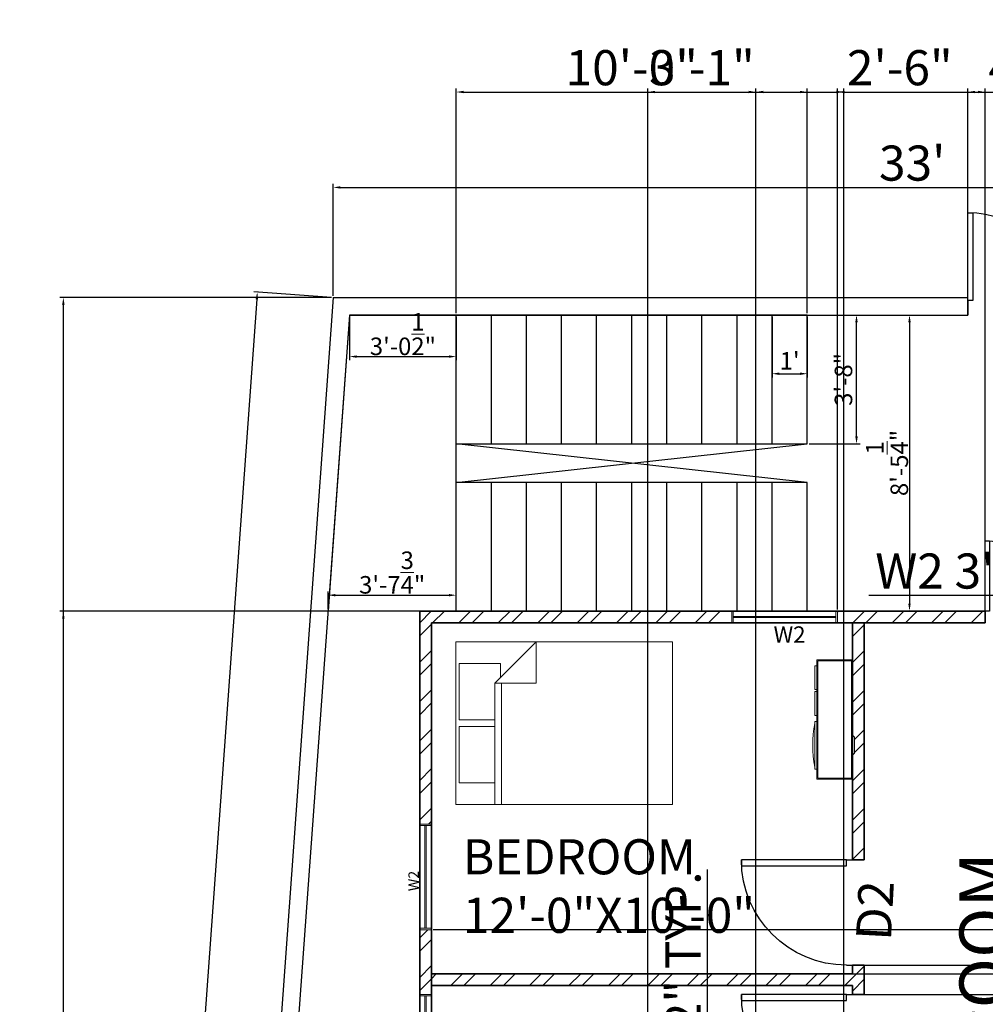
# Model space of a CAD drawing. Units: inches. Extents: x 2242 to 2870, y 1782 to 2635.
# Tile 6 of 7: x 2252 to 2582, y 2299 to 2635. Entities that reach past the tile are written whole.
import ezdxf

# ---------------------------------------------------------------- set-up
doc = ezdxf.new("R2010")
doc.units = ezdxf.units.IN
for name, color, linetype, lineweight in [('A-ANNO-DIMS', 7, 'Continuous', 18), ('A-ANNO-TEXT', 1, 'Continuous', 18), ('A-AREA-IDEN', 1, 'Continuous', 25), ('A-WALL-PATT', 253, 'Continuous', 13), ('C-PROP', 7, 'Continuous', 30), ('doors', 5, 'Continuous', 25), ('furniture', 9, 'Continuous', 18), ('stair case', 6, 'Continuous', 25), ('walls', 7, 'Continuous', 35), ('windows', 72, 'Continuous', 18)]:
    doc.layers.add(name, color=color, linetype=linetype, lineweight=lineweight)
doc.styles.get("Standard").update_dxf_attribs({"font": 'arial.ttf'})
doc.dimstyles.new('ISO-25', dxfattribs={"dimtxt": 12, "dimasz": 2.5, "dimexe": 1.25, "dimexo": 0.625, "dimtad": 1, "dimlunit": 4, "dimtxsty": 'Standard', "dimcen": 2.5, "dimadec": 0, "dimazin": 0, "dimtfac": 1, "dimtmove": 0, "dimatfit": 3, "dimfxl": 1, "dimarcsym": 0})

# ---------------------------------------------------------------- blocks, each defined once
blk = doc.blocks.new('*U2')
for p, q in [((0, 0), (0, -5)), ((30, 0), (30, -5))]:
    blk.add_line(p, q)
blk.add_lwpolyline([(0, 0), (0, 30), (1.75, 30), (1.75, 0)], close=True)
blk.add_arc((0, 0), 30, 0, 90)
blk = doc.blocks.new('Bed - Queen')
for p, q in [((0, -80.00003), (0, 0)), ((0, 0), (59.99999, 0)), ((59.99999, 0), (59.99999, -80.00003)), ((7.99999, -1.2), (28.79998, -1.2)), ((7.99999, -14.4), (7.99999, -1.2)), ((28.79998, -1.2), (28.79998, -14.4)), ((31.19999, -1.2), (51.99999, -1.2)), ((31.19999, -14.4), (31.19999, -1.2)), ((51.99999, -1.2), (51.99999, -16.4)), ((0, -14.4), (44.8, -14.4)), ((59.99999, -29.6), (44.8, -14.4)), ((44.8, -14.4), (44.8, -29.6)), ((44.8, -16.8), (0, -16.8)), ((51.99999, -16.4), (46.79936, -16.4)), ((44.8, -29.6), (59.99999, -29.6)), ((59.99999, -80.00003), (0, -80.00003))]:
    blk.add_line(p, q)
blk = doc.blocks.new('Entertainment Center')
for p, q in [((-4, 0), (-5, -1)), ((4, 0), (-4, 0)), ((5, -1), (4, 0)), ((-17, -19), (-17, -1)), ((-17, -1), (43, -1)), ((-16.5, -18.5), (-16.5, -1.5)), ((-16.5, -1.5), (42.5, -1.5)), ((42.5, -1.5), (42.5, -18.5)), ((43, -1), (43, -19)), ((43, -19), (-17, -19)), ((42.5, -18.5), (-16.5, -18.5)), ((-12, -20), (-12, -19)), ((12, -19), (12, -20)), ((15, -20), (15, -19)), ((27, -19), (27, -20)), ((28, -20), (28, -19)), ((40, -19), (40, -20)), ((12, -20), (-12, -20)), ((27, -20), (15, -20)), ((40, -20), (28, -20))]:
    blk.add_line(p, q)
blk.add_arc((0, 40), 61, 259.6111, 280.3889)
blk = doc.blocks.new('*D15')
at = {"layer": 'A-ANNO-DIMS', "color": 0, "lineweight": -2, "transparency": 16777216}
for p, q in [((2359.16, 2540.96), (2359.16, 2579.23)), ((2755.16, 2540.96), (2755.16, 2579.23)), ((2361.66, 2577.98), (2752.66, 2577.98))]:
    blk.add_line(p, q, dxfattribs=at)
at = {"layer": 'A-ANNO-DIMS', "color": 0, "transparency": 16777216}
for points in [[(2361.66, 2578.39), (2361.66, 2577.56), (2359.16, 2577.98)], [(2752.66, 2578.39), (2752.66, 2577.56), (2755.16, 2577.98)]]:
    blk.add_solid(points, dxfattribs=at)
at = {"layer": 'Defpoints', "color": 0, "transparency": 16777216}
for p in [(2755.16, 2577.98), (2359.16, 2540.33), (2755.16, 2540.33)]:
    blk.add_point(p, dxfattribs=at)
at = {"layer": 'A-ANNO-DIMS', "color": 0, "transparency": 16777216, "insert": (2557.16, 2584.73), "char_height": 12, "attachment_point": 5}
blk.add_mtext("33'", dxfattribs=at)
blk = doc.blocks.new('*D16')
at = {"layer": 'A-ANNO-DIMS', "color": 0, "lineweight": -2, "transparency": 16777216}
for p, q in [((2358.54, 2540.38), (2331.98, 2542.3)), ((2333.04, 2539.72), (2282.38, 1840.55)), ((2307.51, 1836.23), (2280.95, 1838.15))]:
    blk.add_line(p, q, dxfattribs=at)
at = {"layer": 'A-ANNO-DIMS', "color": 0, "transparency": 16777216}
for points in [[(2332.63, 2539.75), (2333.46, 2539.69), (2333.22, 2542.21)], [(2281.96, 1840.58), (2282.79, 1840.52), (2282.2, 1838.06)]]:
    blk.add_solid(points, dxfattribs=at)
at = {"layer": 'Defpoints', "color": 0, "transparency": 16777216}
for p in [(2359.16, 2540.33), (2282.2, 1838.06), (2308.14, 1836.18)]:
    blk.add_point(p, dxfattribs=at)
at = {"layer": 'A-ANNO-DIMS', "color": 0, "transparency": 16777216, "insert": (2300.98, 2190.63), "char_height": 12, "attachment_point": 5, "rotation": 85.8553}
blk.add_mtext('58\'-10"', dxfattribs=at)
blk = doc.blocks.new('*D23')
at = {"layer": 'A-ANNO-DIMS', "color": 0, "lineweight": -2, "transparency": 16777216}
for p, q in [((2509.25, 2533.71), (2509.25, 2513.03)), ((2521.25, 2533.71), (2521.25, 2513.03)), ((2511.75, 2514.28), (2518.75, 2514.28))]:
    blk.add_line(p, q, dxfattribs=at)
at = {"layer": 'A-ANNO-DIMS', "color": 0, "transparency": 16777216}
for points in [[(2511.75, 2514.7), (2511.75, 2513.86), (2509.25, 2514.28)], [(2518.75, 2514.7), (2518.75, 2513.86), (2521.25, 2514.28)]]:
    blk.add_solid(points, dxfattribs=at)
at = {"layer": 'Defpoints', "color": 0, "transparency": 16777216}
for p in [(2509.25, 2534.33), (2521.25, 2534.33), (2521.25, 2514.28)]:
    blk.add_point(p, dxfattribs=at)
at = {"layer": 'A-ANNO-DIMS', "color": 0, "transparency": 16777216, "insert": (2515.25, 2517.92), "char_height": 6, "attachment_point": 5}
blk.add_mtext("1'", dxfattribs=at)
blk = doc.blocks.new('*D24')
at = {"layer": 'A-ANNO-DIMS', "color": 0, "lineweight": -2, "transparency": 16777216}
for p, q in [((2521.88, 2534.33), (2539.37, 2534.33)), ((2538.12, 2492.83), (2538.12, 2531.83)), ((2521.88, 2490.33), (2539.37, 2490.33))]:
    blk.add_line(p, q, dxfattribs=at)
at = {"layer": 'A-ANNO-DIMS', "color": 0, "transparency": 16777216}
for points in [[(2537.7, 2531.83), (2538.54, 2531.83), (2538.12, 2534.33)], [(2537.7, 2492.83), (2538.54, 2492.83), (2538.12, 2490.33)]]:
    blk.add_solid(points, dxfattribs=at)
at = {"layer": 'Defpoints', "color": 0, "transparency": 16777216}
for p in [(2521.25, 2534.33), (2538.12, 2534.33), (2521.25, 2490.33)]:
    blk.add_point(p, dxfattribs=at)
at = {"layer": 'A-ANNO-DIMS', "color": 0, "transparency": 16777216, "insert": (2534.43, 2512.33), "char_height": 6, "attachment_point": 5, "rotation": 90}
blk.add_mtext('3\'-8"', dxfattribs=at)
blk = doc.blocks.new('*D25')
at = {"layer": 'A-ANNO-DIMS', "color": 0, "lineweight": -2, "transparency": 16777216}
for p, q in [((2521.88, 2534.33), (2557.49, 2534.33)), ((2556.24, 2531.83), (2556.24, 2435.7)), ((2521.88, 2433.2), (2557.49, 2433.2))]:
    blk.add_line(p, q, dxfattribs=at)
at = {"layer": 'A-ANNO-DIMS', "color": 0, "transparency": 16777216}
for points in [[(2555.82, 2531.83), (2556.65, 2531.83), (2556.24, 2534.33)], [(2555.82, 2435.7), (2556.65, 2435.7), (2556.24, 2433.2)]]:
    blk.add_solid(points, dxfattribs=at)
at = {"layer": 'Defpoints', "color": 0, "transparency": 16777216}
for p in [(2521.25, 2534.33), (2521.25, 2433.2), (2556.24, 2433.2)]:
    blk.add_point(p, dxfattribs=at)
at = {"layer": 'A-ANNO-DIMS', "color": 0, "transparency": 16777216, "insert": (2548.55, 2483.77), "char_height": 6, "attachment_point": 5, "rotation": 90}
blk.add_mtext('8\'-5{\\H1x;\\S1/4;}"', dxfattribs=at)
blk = doc.blocks.new('*D26')
at = {"layer": 'A-ANNO-DIMS', "color": 0, "lineweight": -2, "transparency": 16777216}
for p, q in [((2357.42, 2433.83), (2357.42, 2439.82)), ((2359.92, 2438.57), (2398.75, 2438.57)), ((2401.25, 2433.83), (2401.25, 2439.82))]:
    blk.add_line(p, q, dxfattribs=at)
at = {"layer": 'A-ANNO-DIMS', "color": 0, "transparency": 16777216}
for points in [[(2359.92, 2438.98), (2359.92, 2438.15), (2357.42, 2438.57)], [(2398.75, 2438.98), (2398.75, 2438.15), (2401.25, 2438.57)]]:
    blk.add_solid(points, dxfattribs=at)
at = {"layer": 'Defpoints', "color": 0, "transparency": 16777216}
for p in [(2401.25, 2438.57), (2357.42, 2433.2), (2401.25, 2433.2)]:
    blk.add_point(p, dxfattribs=at)
at = {"layer": 'A-ANNO-DIMS', "color": 0, "transparency": 16777216, "insert": (2379.33, 2446.31), "char_height": 6, "attachment_point": 5}
blk.add_mtext('3\'-7{\\H1x;\\S3/4;}"', dxfattribs=at)
blk = doc.blocks.new('*D27')
at = {"layer": 'A-ANNO-DIMS', "color": 0, "lineweight": -2, "transparency": 16777216}
for p, q in [((2364.74, 2533.71), (2364.74, 2518.89)), ((2401.25, 2533.71), (2401.25, 2518.89)), ((2367.24, 2520.14), (2398.75, 2520.14))]:
    blk.add_line(p, q, dxfattribs=at)
at = {"layer": 'A-ANNO-DIMS', "color": 0, "transparency": 16777216}
for points in [[(2367.24, 2520.55), (2367.24, 2519.72), (2364.74, 2520.14)], [(2398.75, 2520.55), (2398.75, 2519.72), (2401.25, 2520.14)]]:
    blk.add_solid(points, dxfattribs=at)
at = {"layer": 'Defpoints', "color": 0, "transparency": 16777216}
for p in [(2364.74, 2534.33), (2401.25, 2534.33), (2401.25, 2520.14)]:
    blk.add_point(p, dxfattribs=at)
at = {"layer": 'A-ANNO-DIMS', "color": 0, "transparency": 16777216, "insert": (2383, 2527.84), "char_height": 6, "attachment_point": 5}
blk.add_mtext('3\'-0{\\H1x;\\S1/2;}"', dxfattribs=at)
blk = doc.blocks.new('WIN-W2-36IN')
for p, q in [((0, 4), (36.12, 4)), ((0, 0), (0, 4)), ((0.5, 0), (0.5, 4)), ((35.62, 4), (35.62, 0)), ((36.12, 4), (36.12, 0)), ((36.12, 0), (0, 0)), ((0.5, 2.2), (35.62, 2.2)), ((0.5, 1.8), (35.62, 1.8))]:
    blk.add_line(p, q)
blk = doc.blocks.new('*D33')
at = {"layer": 'A-ANNO-DIMS', "color": 0, "lineweight": -2, "transparency": 16777216}
for p, q in [((2649.56, 2438.51), (2542.37, 2438.51)), ((2649.56, 2433.72), (2649.56, 2439.76)), ((2683.18, 2438.51), (2652.06, 2438.51)), ((2685.68, 2433.72), (2685.68, 2439.76))]:
    blk.add_line(p, q, dxfattribs=at)
at = {"layer": 'A-ANNO-DIMS', "color": 0, "transparency": 16777216}
for points in [[(2652.06, 2438.93), (2652.06, 2438.1), (2649.56, 2438.51)], [(2683.18, 2438.93), (2683.18, 2438.1), (2685.68, 2438.51)]]:
    blk.add_solid(points, dxfattribs=at)
at = {"layer": 'Defpoints', "color": 0, "transparency": 16777216}
for p in [(2649.56, 2438.51), (2649.56, 2433.1), (2685.68, 2433.1)]:
    blk.add_point(p, dxfattribs=at)
at = {"layer": 'A-ANNO-DIMS', "color": 0, "transparency": 16777216, "insert": (2594.72, 2445.27), "char_height": 12, "attachment_point": 5}
blk.add_mtext('W2 3\'-0" TYP.', dxfattribs=at)
blk = doc.blocks.new('*D40')
at = {"layer": 'A-ANNO-DIMS', "color": 0, "lineweight": -2, "transparency": 16777216}
for p, q in [((2487.18, 2239.45), (2487.18, 2344.79)), ((2476.69, 2239.45), (2488.43, 2239.45)), ((2487.18, 2186.37), (2487.18, 2236.95)), ((2476.69, 2183.87), (2488.43, 2183.87))]:
    blk.add_line(p, q, dxfattribs=at)
at = {"layer": 'A-ANNO-DIMS', "color": 0, "transparency": 16777216}
for points in [[(2486.76, 2236.95), (2487.59, 2236.95), (2487.18, 2239.45)], [(2486.76, 2186.37), (2487.59, 2186.37), (2487.18, 2183.87)]]:
    blk.add_solid(points, dxfattribs=at)
at = {"layer": 'Defpoints', "color": 0, "transparency": 16777216}
for p in [(2476.06, 2239.45), (2487.18, 2239.45), (2476.06, 2183.87)]:
    blk.add_point(p, dxfattribs=at)
at = {"layer": 'A-ANNO-DIMS', "color": 0, "transparency": 16777216, "insert": (2480.35, 2293.37), "char_height": 12, "attachment_point": 5, "rotation": 90}
blk.add_mtext('4\'-7 1/2" TYP.', dxfattribs=at)
blk = doc.blocks.new('*D55')
at = {"layer": 'A-ANNO-DIMS', "color": 0, "lineweight": -2, "transparency": 16777216}
for p, q in [((2358.54, 2540.33), (2265.64, 2540.33)), ((2266.89, 1838.68), (2266.89, 2537.83)), ((2307.51, 1836.18), (2265.64, 1836.18))]:
    blk.add_line(p, q, dxfattribs=at)
at = {"layer": 'A-ANNO-DIMS', "color": 0, "transparency": 16777216}
for points in [[(2266.47, 2537.83), (2267.3, 2537.83), (2266.89, 2540.33)], [(2266.47, 1838.68), (2267.3, 1838.68), (2266.89, 1836.18)]]:
    blk.add_solid(points, dxfattribs=at)
at = {"layer": 'Defpoints', "color": 0, "transparency": 16777216}
for p in [(2266.89, 2540.33), (2359.16, 2540.33), (2308.14, 1836.18)]:
    blk.add_point(p, dxfattribs=at)
at = {"layer": 'A-ANNO-DIMS', "color": 0, "transparency": 16777216, "insert": (2260.13, 2188.26), "char_height": 12, "attachment_point": 5, "rotation": 90}
blk.add_mtext('58\'-8"', dxfattribs=at)
blk = doc.blocks.new('*D58')
at = {"layer": 'A-ANNO-DIMS', "color": 0, "lineweight": -2, "transparency": 16777216}
for p, q in [((2388.12, 2433.1), (2265.64, 2433.1)), ((2266.89, 1899.6), (2266.89, 2430.6)), ((2388.12, 1897.1), (2265.64, 1897.1))]:
    blk.add_line(p, q, dxfattribs=at)
at = {"layer": 'A-ANNO-DIMS', "color": 0, "transparency": 16777216}
for points in [[(2266.47, 2430.6), (2267.3, 2430.6), (2266.89, 2433.1)], [(2266.47, 1899.6), (2267.3, 1899.6), (2266.89, 1897.1)]]:
    blk.add_solid(points, dxfattribs=at)
at = {"layer": 'Defpoints', "color": 0, "transparency": 16777216}
for p in [(2266.89, 2433.1), (2388.74, 2433.1), (2388.74, 1897.1)]:
    blk.add_point(p, dxfattribs=at)
at = {"layer": 'A-ANNO-DIMS', "color": 0, "transparency": 16777216, "insert": (2260.13, 2165.1), "char_height": 12, "attachment_point": 5, "rotation": 90}
blk.add_mtext('44\'-8"', dxfattribs=at)
blk = doc.blocks.new('*D59')
at = {"layer": 'A-ANNO-DIMS', "color": 0, "lineweight": -2, "transparency": 16777216}
for p, q in [((2576.16, 2540.96), (2576.16, 2611.83)), ((2578.66, 2610.58), (2633.66, 2610.58)), ((2636.16, 2540.96), (2636.16, 2611.83))]:
    blk.add_line(p, q, dxfattribs=at)
at = {"layer": 'A-ANNO-DIMS', "color": 0, "transparency": 16777216}
for points in [[(2578.66, 2611), (2578.66, 2610.17), (2576.16, 2610.58)], [(2633.66, 2611), (2633.66, 2610.17), (2636.16, 2610.58)]]:
    blk.add_solid(points, dxfattribs=at)
at = {"layer": 'Defpoints', "color": 0, "transparency": 16777216}
for p in [(2636.16, 2610.58), (2576.16, 2540.33), (2636.16, 2540.33)]:
    blk.add_point(p, dxfattribs=at)
at = {"layer": 'A-ANNO-DIMS', "color": 0, "transparency": 16777216, "insert": (2606.16, 2617.34), "char_height": 12, "attachment_point": 5}
blk.add_mtext('5\'-0"', dxfattribs=at)
blk = doc.blocks.new('*D62')
at = {"layer": 'A-ANNO-DIMS', "color": 0, "lineweight": -2, "transparency": 16777216}
for p, q in [((2537.37, 2302.1), (2797.66, 2302.1)), ((2796.41, 2299.6), (2796.41, 2268.6)), ((2537.37, 2266.1), (2797.66, 2266.1))]:
    blk.add_line(p, q, dxfattribs=at)
at = {"layer": 'A-ANNO-DIMS', "color": 0, "transparency": 16777216}
for points in [[(2796, 2299.6), (2796.83, 2299.6), (2796.41, 2302.1)], [(2796, 2268.6), (2796.83, 2268.6), (2796.41, 2266.1)]]:
    blk.add_solid(points, dxfattribs=at)
at = {"layer": 'Defpoints', "color": 0, "transparency": 16777216}
for p in [(2536.74, 2302.1), (2536.74, 2266.1), (2796.41, 2266.1)]:
    blk.add_point(p, dxfattribs=at)
at = {"layer": 'A-ANNO-DIMS', "color": 0, "transparency": 16777216, "insert": (2789.66, 2284.1), "char_height": 12, "attachment_point": 5, "rotation": 90}
blk.add_mtext('3\'-0"', dxfattribs=at)
blk = doc.blocks.new('*D63')
at = {"layer": 'A-ANNO-DIMS', "color": 0, "lineweight": -2, "transparency": 16777216}
for p, q in [((2503.74, 2161.72), (2503.74, 2611.83)), ((2506.24, 2610.58), (2531.24, 2610.58)), ((2533.74, 2161.72), (2533.74, 2611.83)), ((2533.74, 2610.58), (2569.6, 2610.58))]:
    blk.add_line(p, q, dxfattribs=at)
at = {"layer": 'A-ANNO-DIMS', "color": 0, "transparency": 16777216}
for points in [[(2506.24, 2611), (2506.24, 2610.17), (2503.74, 2610.58)], [(2531.24, 2611), (2531.24, 2610.17), (2533.74, 2610.58)]]:
    blk.add_solid(points, dxfattribs=at)
at = {"layer": 'Defpoints', "color": 0, "transparency": 16777216}
for p in [(2533.74, 2610.58), (2503.74, 2161.1), (2533.74, 2161.1)]:
    blk.add_point(p, dxfattribs=at)
at = {"layer": 'A-ANNO-DIMS', "color": 0, "transparency": 16777216, "insert": (2552.92, 2617.34), "char_height": 12, "attachment_point": 5}
blk.add_mtext('2\'-6"', dxfattribs=at)
blk = doc.blocks.new('*D71')
at = {"layer": 'A-ANNO-DIMS', "color": 0, "lineweight": -2, "transparency": 16777216}
for p, q in [((2531.58, 2433.72), (2531.58, 2611.83)), ((2534.08, 2610.58), (2579.66, 2610.58)), ((2582.16, 2433.72), (2582.16, 2611.83)), ((2582.16, 2610.58), (2646.26, 2610.58))]:
    blk.add_line(p, q, dxfattribs=at)
at = {"layer": 'A-ANNO-DIMS', "color": 0, "transparency": 16777216}
for points in [[(2534.08, 2611), (2534.08, 2610.17), (2531.58, 2610.58)], [(2579.66, 2611), (2579.66, 2610.17), (2582.16, 2610.58)]]:
    blk.add_solid(points, dxfattribs=at)
at = {"layer": 'Defpoints', "color": 0, "transparency": 16777216}
for p in [(2582.16, 2610.58), (2531.58, 2433.1), (2582.16, 2433.1)]:
    blk.add_point(p, dxfattribs=at)
at = {"layer": 'A-ANNO-DIMS', "color": 0, "transparency": 16777216, "insert": (2615.46, 2617.41), "char_height": 12, "attachment_point": 5}
blk.add_mtext('4\'-2 1/2"', dxfattribs=at)
blk = doc.blocks.new('*D79')
at = {"layer": 'A-ANNO-DIMS', "color": 0, "lineweight": -2, "transparency": 16777216}
for p, q in [((2796.41, 2324.23), (2796.41, 2358.75)), ((2393.37, 2324.23), (2797.66, 2324.23)), ((2796.41, 2311.6), (2796.41, 2321.73)), ((2393.37, 2309.1), (2797.66, 2309.1))]:
    blk.add_line(p, q, dxfattribs=at)
at = {"layer": 'A-ANNO-DIMS', "color": 0, "transparency": 16777216}
for points in [[(2796, 2321.73), (2796.83, 2321.73), (2796.41, 2324.23)], [(2796, 2311.6), (2796.83, 2311.6), (2796.41, 2309.1)]]:
    blk.add_solid(points, dxfattribs=at)
at = {"layer": 'Defpoints', "color": 0, "transparency": 16777216}
for p in [(2392.74, 2324.23), (2796.41, 2324.23), (2392.74, 2309.1)]:
    blk.add_point(p, dxfattribs=at)
at = {"layer": 'A-ANNO-DIMS', "color": 0, "transparency": 16777216, "insert": (2789.66, 2342.74), "char_height": 12, "attachment_point": 5, "rotation": 90}
blk.add_mtext('1\'-3"', dxfattribs=at)
blk = doc.blocks.new('*D83')
at = {"layer": 'A-ANNO-DIMS', "color": 0, "lineweight": -2, "transparency": 16777216}
for p, q in [((2796.41, 2314.6), (2796.41, 2350.25)), ((2537.37, 2312.1), (2797.66, 2312.1)), ((2537.37, 2309.1), (2797.66, 2309.1)), ((2796.41, 2309.1), (2796.41, 2312.1)), ((2796.41, 2306.6), (2796.41, 2304.1))]:
    blk.add_line(p, q, dxfattribs=at)
at = {"layer": 'A-ANNO-DIMS', "color": 0, "transparency": 16777216}
for points in [[(2796, 2314.6), (2796.83, 2314.6), (2796.41, 2312.1)], [(2796, 2306.6), (2796.83, 2306.6), (2796.41, 2309.1)]]:
    blk.add_solid(points, dxfattribs=at)
at = {"layer": 'Defpoints', "color": 0, "transparency": 16777216}
for p in [(2536.74, 2312.1), (2536.74, 2309.1), (2796.41, 2312.1)]:
    blk.add_point(p, dxfattribs=at)
at = {"layer": 'A-ANNO-DIMS', "color": 0, "transparency": 16777216, "insert": (2789.66, 2333.67), "char_height": 12, "attachment_point": 5, "rotation": 90}
blk.add_mtext('0\'-3"', dxfattribs=at)
blk = doc.blocks.new('*D84')
at = {"layer": 'A-ANNO-DIMS', "color": 0, "lineweight": -2, "transparency": 16777216}
for p, q in [((2401.25, 2534.96), (2401.25, 2611.83)), ((2403.75, 2610.58), (2518.75, 2610.58)), ((2521.25, 2534.96), (2521.25, 2611.83))]:
    blk.add_line(p, q, dxfattribs=at)
at = {"layer": 'A-ANNO-DIMS', "color": 0, "transparency": 16777216}
for points in [[(2403.75, 2611), (2403.75, 2610.17), (2401.25, 2610.58)], [(2518.75, 2611), (2518.75, 2610.17), (2521.25, 2610.58)]]:
    blk.add_solid(points, dxfattribs=at)
at = {"layer": 'Defpoints', "color": 0, "transparency": 16777216}
for p in [(2521.25, 2610.58), (2401.25, 2534.33), (2521.25, 2534.33)]:
    blk.add_point(p, dxfattribs=at)
at = {"layer": 'A-ANNO-DIMS', "color": 0, "transparency": 16777216, "insert": (2461.25, 2617.34), "char_height": 12, "attachment_point": 5}
blk.add_mtext('10\'-0"', dxfattribs=at)
blk = doc.blocks.new('*D87')
at = {"layer": 'A-ANNO-DIMS', "color": 0, "lineweight": -2, "transparency": 16777216}
for p, q in [((2466.74, 2157.72), (2466.74, 2611.83)), ((2469.24, 2610.58), (2501.24, 2610.58)), ((2503.74, 2157.72), (2503.74, 2611.83))]:
    blk.add_line(p, q, dxfattribs=at)
at = {"layer": 'A-ANNO-DIMS', "color": 0, "transparency": 16777216}
for points in [[(2469.24, 2611), (2469.24, 2610.17), (2466.74, 2610.58)], [(2501.24, 2611), (2501.24, 2610.17), (2503.74, 2610.58)]]:
    blk.add_solid(points, dxfattribs=at)
at = {"layer": 'Defpoints', "color": 0, "transparency": 16777216}
for p in [(2503.74, 2610.58), (2466.74, 2157.1), (2503.74, 2157.1)]:
    blk.add_point(p, dxfattribs=at)
at = {"layer": 'A-ANNO-DIMS', "color": 0, "transparency": 16777216, "insert": (2485.24, 2617.34), "char_height": 12, "attachment_point": 5}
blk.add_mtext('3\'-1"', dxfattribs=at)

msp = doc.modelspace()

# ---------------------------------------------------------------- hatches: boundary and pattern name
at = {"layer": 'A-WALL-PATT'}
h = msp.add_hatch(dxfattribs=at)
h.set_pattern_fill('ANSI32', color=256)
h.paths.add_polyline_path([(2495.468, 2433.097), (2388.745, 2433.097), (2388.745, 2360.342), (2392.745, 2360.342), (2392.745, 2429.097), (2495.468, 2429.097)])
h = msp.add_hatch(dxfattribs=at)
h.set_pattern_fill('ANSI32', color=256)
h.paths.add_polyline_path([(2582.164, 2433.097), (2531.584, 2433.097), (2531.584, 2429.097), (2582.164, 2429.097)])
h = msp.add_hatch(dxfattribs=at)
h.set_pattern_fill('ANSI32', color=256)
h.paths.add_polyline_path([(2540.745, 2429.097), (2536.745, 2429.097), (2536.745, 2390.661), (2537.424, 2389.981), (2537.424, 2384.547), (2536.745, 2383.867), (2536.745, 2375.715), (2536.745, 2348.097), (2540.745, 2348.097)])
h = msp.add_hatch(dxfattribs=at)
h.set_pattern_fill('ANSI32', color=256)
h.paths.add_polyline_path([(2392.745, 2324.226), (2388.745, 2324.226), (2388.745, 2302.109), (2392.745, 2302.109)])
h = msp.add_hatch(dxfattribs=at)
h.set_pattern_fill('ANSI32', color=256)
h.paths.add_polyline_path([(2540.745, 2312.097), (2536.745, 2312.097), (2536.745, 2309.097), (2392.745, 2309.097), (2392.745, 2305.097), (2536.745, 2305.097), (2536.745, 2302.097), (2540.745, 2302.097), (2540.745, 2305.097)])

# ---------------------------------------------------------------- linework, layer by layer
at = {"layer": 'C-PROP'}
for p, q in [((2359.164, 2540.335), (2308.137, 1836.181)), ((2359.164, 2540.335), (2576.164, 2540.335)), ((2576.164, 2534.335), (2576.164, 2540.335)), ((2364.745, 2534.335), (2314.71, 1843.873)), ((2364.745, 2534.335), (2576.164, 2534.335))]:
    msp.add_line(p, q, dxfattribs=at)
at = {"layer": 'stair case'}
for p, q in [((2364.745, 2534.335), (2357.416, 2433.205)), ((2521.253, 2534.335), (2364.745, 2534.335)), ((2401.253, 2433.097), (2401.253, 2534.335)), ((2413.253, 2490.335), (2413.253, 2534.335)), ((2425.253, 2490.335), (2425.253, 2534.335)), ((2437.253, 2490.335), (2437.253, 2534.335)), ((2449.253, 2490.335), (2449.253, 2534.335)), ((2461.253, 2490.335), (2461.253, 2534.335)), ((2473.253, 2490.335), (2473.253, 2534.335)), ((2485.253, 2490.335), (2485.253, 2534.335)), ((2497.253, 2490.335), (2497.253, 2534.335)), ((2509.253, 2490.335), (2509.253, 2534.335)), ((2521.253, 2490.335), (2521.253, 2534.335)), ((2401.253, 2490.335), (2521.253, 2490.335)), ((2401.253, 2477.097), (2521.253, 2490.335)), ((2521.253, 2477.097), (2401.253, 2490.335)), ((2521.253, 2477.097), (2401.253, 2477.097)), ((2413.253, 2433.097), (2413.253, 2477.097)), ((2425.253, 2433.097), (2425.253, 2477.097)), ((2437.253, 2433.097), (2437.253, 2477.097)), ((2449.253, 2433.097), (2449.253, 2477.097)), ((2461.253, 2433.097), (2461.253, 2477.097)), ((2473.253, 2433.097), (2473.253, 2477.097)), ((2485.253, 2433.097), (2485.253, 2477.097)), ((2497.253, 2433.097), (2497.253, 2477.097)), ((2509.253, 2433.097), (2509.253, 2477.097)), ((2521.253, 2433.097), (2521.253, 2477.097)), ((2357.416, 2433.205), (2521.253, 2433.205))]:
    msp.add_line(p, q, dxfattribs=at)
at = {"layer": 'walls'}
for p, q in [((2388.745, 1957.097), (2388.745, 2433.097)), ((2582.164, 2433.097), (2388.745, 2433.097)), ((2582.164, 2429.097), (2582.164, 2433.097)), ((2392.745, 1961.097), (2392.745, 2429.097)), ((2582.164, 2429.097), (2392.745, 2429.097)), ((2536.745, 2348.097), (2536.745, 2429.097)), ((2540.745, 2348.097), (2540.745, 2429.097)), ((2536.745, 2348.097), (2540.745, 2348.097)), ((2536.745, 2309.097), (2392.745, 2309.097)), ((2540.745, 2312.097), (2536.745, 2312.097)), ((2536.745, 2309.097), (2536.745, 2312.097)), ((2540.745, 2309.097), (2540.745, 2312.097)), ((2540.745, 2302.097), (2540.745, 2312.097)), ((2536.745, 2305.097), (2392.745, 2305.097)), ((2536.745, 2302.097), (2536.745, 2305.097)), ((2540.745, 2305.097), (2540.745, 2302.097)), ((2540.745, 2302.097), (2536.745, 2302.097))]:
    msp.add_line(p, q, dxfattribs=at)

# ---------------------------------------------------------------- block references
at = {"layer": 'doors'}
msp.add_blockref('*U2', (2576.164, 2539.335), dxfattribs=at)
at = {"layer": 'doors', "xscale": 0.8, "yscale": 0.8, "zscale": 0.8}
msp.add_blockref('*U2', (2582.164, 2433.097), dxfattribs=at)
at = {"layer": 'doors', "xscale": -1.199999999999999, "yscale": 1.199999999999999, "zscale": 1.199999999999999, "rotation": 90}
for p in [(2534.745, 2348.097), (2534.745, 2302.097)]:
    msp.add_blockref('*U2', p, dxfattribs=at)
at = {"layer": 'furniture'}
for name, p, xscale, yscale, zscale, rotation in [('Bed - Queen', (2401.132, 2367.03), 0.9262549739508827, 0.9262549739508827, 0.9262549739508827, 90), ('Entertainment Center', (2537.424, 2387.264), -0.6793374069686555, 0.6793374069686555, 0.6793374069686555, 270)]:
    msp.add_blockref(name, p, dxfattribs=dict(at, xscale=xscale, yscale=yscale, zscale=zscale, rotation=rotation))
at = {"layer": 'windows'}
msp.add_blockref('WIN-W2-36IN', (2495.468, 2429.097), dxfattribs=at)
for p, rotation in [((2392.745, 2324.226), 89.99999999999586), ((2392.745, 2265.993), 89.99999999999604)]:
    msp.add_blockref('WIN-W2-36IN', p, dxfattribs=dict(at, rotation=rotation))

# ---------------------------------------------------------------- texts
at = {"layer": 'A-ANNO-TEXT', "insert": (2509.759, 2427.906), "char_height": 5.5921, "attachment_point": 1}
msp.add_mtext_dynamic_manual_height_columns('W2', width=0.54422, gutter_width=27.96, heights=[0], dxfattribs=at)
at = {"layer": 'A-ANNO-TEXT', "attachment_point": 1}
for s, width, gutter_width, insert, char_height, rotation in [('W2', 0.34623, 17.788, (2384.903, 2337.386), 3.5576, 90), ('D2', 2.16795, 12.5, (2537.887, 2320.922), 12, 87.02981)]:
    msp.add_mtext_dynamic_manual_height_columns(s, width=width, gutter_width=gutter_width, heights=[0], dxfattribs=dict(at, insert=insert, char_height=char_height, rotation=rotation))
at = {"layer": 'A-AREA-IDEN', "insert": (2403.518, 2355.142), "char_height": 12, "attachment_point": 1}
msp.add_mtext_dynamic_manual_height_columns('BEDROOM\\P12\'-0"X10\'-0"', width=4.3797, gutter_width=12.5, heights=[0], dxfattribs=at)
at = {"layer": 'A-AREA-IDEN', "insert": (2573.308, 2210.091), "char_height": 17.04609, "attachment_point": 1, "rotation": 90}
msp.add_mtext_dynamic_manual_height_columns('LIVINGROOM\\P14\'-3"X27\'-3"', width=6.2214, gutter_width=17.756, heights=[0], dxfattribs=at)

# ---------------------------------------------------------------- dimensions: what is measured, and where the dimension line sits
at = {"layer": 'A-ANNO-DIMS'}
for base, p1, p2, override, picture, middle in [((2582.164, 2610.585), (2531.584, 2433.097), (2582.164, 2433.097), {"dimdec": 1, "dimlfac": 1, "dimrnd": 0, "dimzin": 1, "dimdsep": 46, "dimlunit": 4, "dimfrac": 2}, '*D71', (2615.46, 2617.414)), ((2521.253, 2610.585), (2401.253, 2534.335), (2521.253, 2534.335), {"dimdec": 1, "dimlfac": 1, "dimrnd": 0, "dimzin": 1, "dimdsep": 46, "dimlunit": 4, "dimfrac": 2}, '*D84', (2461.253, 2617.337)), ((2503.745, 2610.585), (2466.745, 2157.097), (2503.745, 2157.097), {"dimdec": 1, "dimlfac": 1, "dimrnd": 0, "dimzin": 1, "dimdsep": 46, "dimlunit": 4, "dimfrac": 2}, '*D87', (2485.245, 2617.341)), ((2533.745, 2610.585), (2503.745, 2161.097), (2533.745, 2161.097), {"dimdec": 1, "dimlfac": 1, "dimrnd": 0, "dimzin": 1, "dimdsep": 46, "dimlunit": 4, "dimfrac": 2}, '*D63', (2552.921, 2617.337)), ((2636.164, 2610.585), (2576.164, 2540.335), (2636.164, 2540.335), {"dimdec": 1, "dimlfac": 1, "dimrnd": 0, "dimzin": 1, "dimdsep": 46, "dimlunit": 4, "dimfrac": 2}, '*D59', (2606.164, 2617.337)), ((2755.164, 2577.978), (2359.164, 2540.335), (2755.164, 2540.335), {"dimclrd": 0, "dimclre": 0, "dimclrt": 0}, '*D15', (2557.164, 2584.734)), ((2401.253, 2520.137), (2364.745, 2534.335), (2401.253, 2534.335), {"dimtxt": 6, "dimclrd": 0, "dimclre": 0, "dimclrt": 0}, '*D27', (2382.999, 2527.84)), ((2521.253, 2514.281), (2509.253, 2534.335), (2521.253, 2534.335), {"dimtxt": 6, "dimclrd": 0, "dimclre": 0, "dimclrt": 0}, '*D23', (2515.253, 2517.918)), ((2401.253, 2438.568), (2357.416, 2433.205), (2401.253, 2433.205), {"dimtxt": 6, "dimclrd": 0, "dimclre": 0, "dimclrt": 0}, '*D26', (2379.334, 2446.312))]:
    dim = msp.add_linear_dim(base=base, p1=p1, p2=p2, dimstyle='ISO-25', override=override, dxfattribs=at)
    dim.commit()
    dim.dimension.update_dxf_attribs({"geometry": picture, "text_midpoint": middle})
dim = msp.add_aligned_dim(p1=(2359.164, 2540.335), p2=(2308.137, 1836.181), distance=-26.007, dimstyle='ISO-25', override={"dimclrd": 0, "dimclre": 0, "dimclrt": 0}, dxfattribs=at)
dim.commit()
dim.dimension.update_dxf_attribs({"geometry": '*D16', "text_midpoint": (2300.976, 2190.626)})
for base, p1, p2, override, picture, middle in [((2266.887, 2540.335), (2308.137, 1836.181), (2359.164, 2540.335), {"dimdec": 1, "dimlfac": 1, "dimrnd": 0, "dimzin": 1, "dimdsep": 46, "dimlunit": 4, "dimfrac": 2}, '*D55', (2260.135, 2188.258)), ((2538.119, 2534.335), (2521.253, 2490.335), (2521.253, 2534.335), {"dimtxt": 6, "dimclrd": 0, "dimclre": 0, "dimclrt": 0}, '*D24', (2534.428, 2512.335)), ((2556.238, 2433.205), (2521.253, 2534.335), (2521.253, 2433.205), {"dimtxt": 6, "dimclrd": 0, "dimclre": 0, "dimclrt": 0}, '*D25', (2548.55, 2483.77)), ((2266.887, 2433.097), (2388.745, 1897.097), (2388.745, 2433.097), {"dimdec": 1, "dimlfac": 1, "dimrnd": 0, "dimzin": 1, "dimdsep": 46, "dimlunit": 4, "dimfrac": 2}, '*D58', (2260.135, 2165.097)), ((2796.414, 2324.226), (2392.745, 2309.097), (2392.745, 2324.226), {"dimdec": 1, "dimlfac": 1, "dimrnd": 0, "dimzin": 1, "dimdsep": 46, "dimlunit": 4, "dimfrac": 2}, '*D79', (2789.658, 2342.736)), ((2796.414, 2312.097), (2536.745, 2309.097), (2536.745, 2312.097), {"dimdec": 1, "dimlfac": 1, "dimrnd": 0, "dimzin": 1, "dimdsep": 46, "dimlunit": 4, "dimfrac": 2}, '*D83', (2789.658, 2333.672)), ((2796.414, 2266.097), (2536.745, 2302.097), (2536.745, 2266.097), {"dimdec": 1, "dimlfac": 1, "dimrnd": 0, "dimzin": 1, "dimdsep": 46, "dimlunit": 4, "dimfrac": 2}, '*D62', (2789.658, 2284.097))]:
    dim = msp.add_linear_dim(base=base, p1=p1, p2=p2, angle=90, dimstyle='ISO-25', override=override, dxfattribs=at)
    dim.commit()
    dim.dimension.update_dxf_attribs({"geometry": picture, "text_midpoint": middle})
for base, p1, p2, angle, text, picture, middle in [((2649.562, 2438.515), (2685.678, 2433.097), (2649.562, 2433.097), 180, 'W2 <> TYP.', '*D33', (2594.716, 2445.271)), ((2487.178, 2239.449), (2476.063, 2183.874), (2476.063, 2239.449), 90, '<> TYP.', '*D40', (2480.349, 2293.369))]:
    dim = msp.add_linear_dim(base=base, p1=p1, p2=p2, angle=angle, text=text, dimstyle='ISO-25', override={"dimdec": 1, "dimlfac": 1, "dimrnd": 0, "dimzin": 1, "dimdsep": 46, "dimlunit": 4, "dimfrac": 2}, dxfattribs=at)
    dim.commit()
    dim.dimension.update_dxf_attribs({"geometry": picture, "text_midpoint": middle})

doc.saveas('drawing.dxf')
